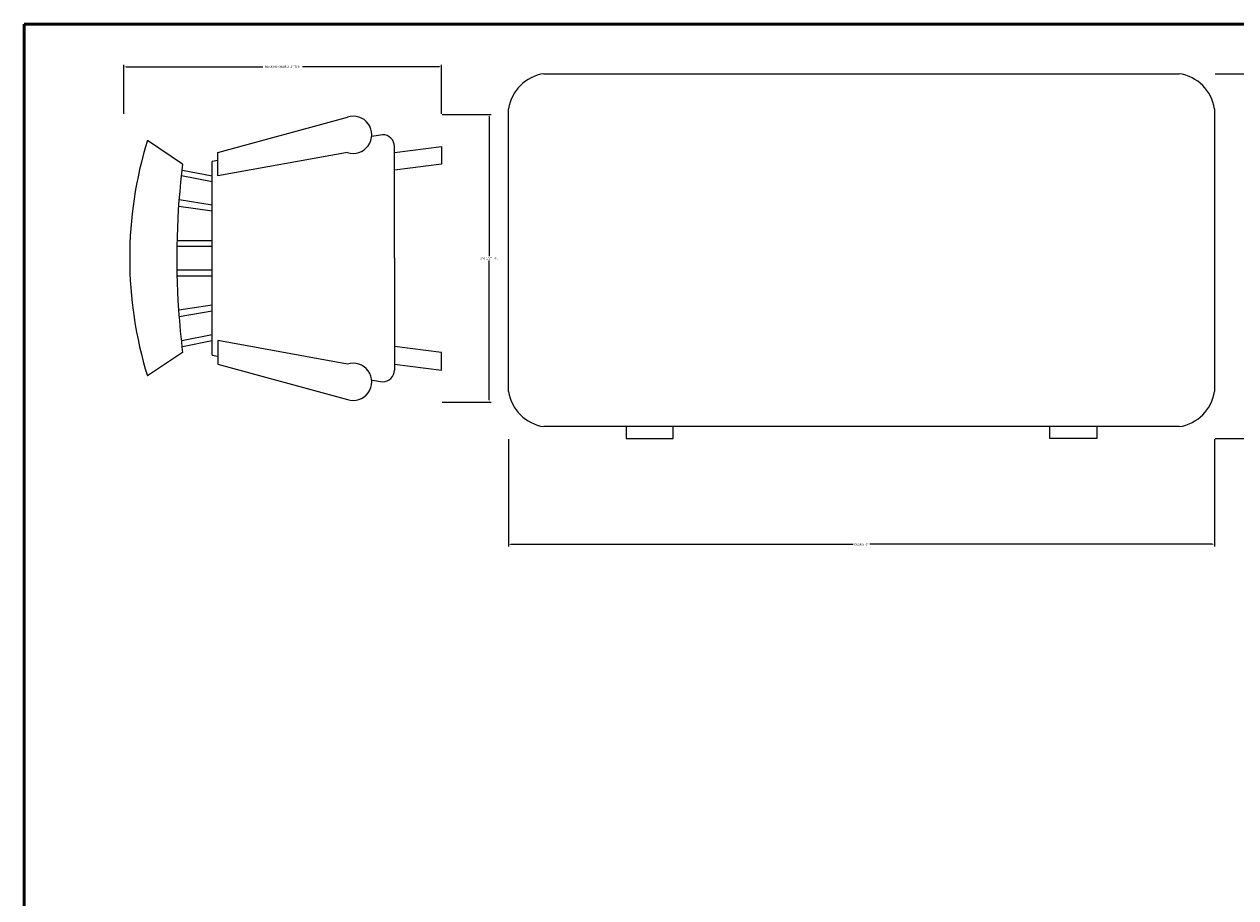
# Model space of a CAD drawing. Units: inches. Extents: x -105 to 1196, y -792 to 119.
# Tile 20 of 23: x 324 to 427, y -199 to -125. Entities that reach past the tile are written whole.
import ezdxf

# ---------------------------------------------------------------- set-up
doc = ezdxf.new("R2010")
doc.units = ezdxf.units.IN
doc.header["$MEASUREMENT"] = 0
for name, color, linetype, lineweight in [('A-ANNO-DIMS', 2, 'Continuous', 18), ('A-FURN', 8, 'Continuous', 18), ('A-WALL', 3, 'Continuous', 50)]:
    doc.layers.add(name, color=color, linetype=linetype, lineweight=lineweight)
doc.styles.get("Standard").update_dxf_attribs({"font": 'arial.ttf'})
doc.dimstyles.get("Standard").update_dxf_attribs({"dimtxt": 0.18, "dimasz": 0.18, "dimexe": 0.18, "dimexo": 0.0625, "dimgap": 0.09, "dimtad": 0, "dimtih": 1, "dimtoh": 1, "dimdec": 1, "dimzin": 0, "dimdsep": 46, "dimlunit": 4, "dimtxsty": 'Standard', "dimcen": 0.09, "dimadec": 0, "dimazin": 0, "dimtfac": 1, "dimtdec": 1, "dimtofl": 0, "dimtmove": 0, "dimatfit": 3, "dimfxl": 1, "dimtolj": 1, "dimtzin": 0, "dimarcsym": 0})

# ---------------------------------------------------------------- blocks, each defined once
blk = doc.blocks.new('Desk - 30 x 60 in.')
for p, q in [((-26.999995, 0), (26.999995, 0)), ((-29.999995, -27), (-29.999995, -3)), ((29.999995, -3), (29.999995, -27)), ((26.999995, -30), (-26.999995, -30)), ((-20.000005, -30), (-20.000005, -31)), ((-16.000005, -31), (-16.000005, -30)), ((15.999995, -31), (15.999995, -30)), ((19.999995, -30), (19.999995, -31)), ((-20.000005, -31), (-16.000005, -31)), ((19.999995, -31), (15.999995, -31))]:
    blk.add_line(p, q)
for centre, start, end in [((-26.499995, -3.5), 98.1301, 171.8699), ((26.499995, -3.5), 8.130102, 81.8699), ((-26.499995, -26.5), 188.1301, 261.8699), ((26.499995, -26.5), 278.1301, 351.8699)]:
    blk.add_arc(centre, 3.535534, start, end)
blk = doc.blocks.new('Chair - Rocking')
for p, q in [((-8, -4.5), (-10, -1.5)), ((8, -4.5), (10, -1.5)), ((-1.5, -4.05012), (-1.5, -7)), ((-1, -7), (-1, -4.05012)), ((1, -7), (1, -4.04655)), ((1.5, -4.05012), (1.5, -7)), ((-7.5, -4.5), (-7, -7)), ((-6.5, -7), (-7.02225, -4.43)), ((-4.5, -7), (-4.96674, -4.19951)), ((-4, -7), (-4.40532, -4.16272)), ((4, -7), (4.40187, -4.18694)), ((4.5, -7), (4.96761, -4.19437)), ((6.5, -7), (7, -4.4057)), ((7.5, -4.5), (7, -7)), ((-8.23428, -6.99939), (-8.3093, -7.47958)), ((-8.23041, -7), (8.23915, -7)), ((8.31071, -7.48854), (8.23449, -7.00073)), ((-9, -7.5), (-12, -18.49999)), ((-7, -7.5), (-9, -7.5)), ((-9, -18.49999), (-7, -7.5)), ((7, -7.5), (9, -7.5)), ((9, -18.49999), (7, -7.5)), ((9, -7.5), (12, -18.49999)), ((10.5, -21.49999), (10.3575, -20.58798)), ((-10.36644, -20.64523), (-10.5, -21.49999)), ((-9, -22.49999), (-9.5, -26.49999)), ((0, -22.49999), (-9.5, -22.49999)), ((-8, -26.49999), (-7.5, -22.49999)), ((0, -22.49999), (9.5, -22.49999)), ((8, -26.49999), (7.5, -22.49999)), ((9, -22.49999), (9.5, -26.49999)), ((-9.5, -26.49999), (-8, -26.49999)), ((9.5, -26.49999), (8, -26.49999))]:
    blk.add_line(p, q)
for centre, radius, start, end in [((0, -34.08333), 34.08333, 72.93847, 107.0615), ((0, -68.25004), 64.25, 82.84733, 93.92211), ((0, -68.25004), 64.25, 93.92211, 97.15267), ((-10.5, -18.99999), 1.58114, 161.5651, 18.43495), ((10.5, -18.99999), 1.58114, 161.5651, 18.43495), ((-9.5, -21.49999), 1, 180, 270), ((9.5, -21.49999), 1, 270, 0)]:
    blk.add_arc(centre, radius, start, end)
blk = doc.blocks.new('*D65')
at = {"layer": 'A-ANNO-DIMS', "color": 0, "lineweight": -2, "transparency": 16777216}
for p, q in [((332.21, -132.84), (332.21, -128.67)), ((359.21, -132.84), (359.21, -128.67)), ((332.39, -128.85), (344.03, -128.85)), ((359.03, -128.85), (347.4, -128.85))]:
    blk.add_line(p, q, dxfattribs=at)
at = {"layer": 'A-ANNO-DIMS', "color": 0, "transparency": 16777216}
for points in [[(332.39, -128.82), (332.39, -128.88), (332.21, -128.85)], [(359.03, -128.82), (359.03, -128.88), (359.21, -128.85)]]:
    blk.add_solid(points, dxfattribs=at)
at = {"layer": 'Defpoints', "color": 0, "transparency": 16777216}
for p in [(332.21, -128.85), (332.21, -132.9), (359.21, -132.9)]:
    blk.add_point(p, dxfattribs=at)
at = {"layer": 'A-ANNO-DIMS', "color": 0, "transparency": 16777216, "insert": (345.71, -128.85), "char_height": 0.18, "attachment_point": 5}
blk.add_mtext('\\A1;ROCKING CHAIR 2\'-3" TYP.', dxfattribs=at)
blk = doc.blocks.new('*D66')
at = {"layer": 'A-ANNO-DIMS', "color": 0, "lineweight": -2, "transparency": 16777216}
for p, q in [((359.28, -132.9), (363.44, -132.9)), ((363.26, -133.08), (363.26, -144.94)), ((363.26, -157.16), (363.26, -145.3)), ((359.28, -157.34), (363.44, -157.34))]:
    blk.add_line(p, q, dxfattribs=at)
at = {"layer": 'A-ANNO-DIMS', "color": 0, "transparency": 16777216}
for points in [[(363.23, -133.08), (363.29, -133.08), (363.26, -132.9)], [(363.23, -157.16), (363.29, -157.16), (363.26, -157.34)]]:
    blk.add_solid(points, dxfattribs=at)
at = {"layer": 'Defpoints', "color": 0, "transparency": 16777216}
for p in [(359.21, -132.9), (363.26, -132.9), (359.21, -157.34)]:
    blk.add_point(p, dxfattribs=at)
at = {"layer": 'A-ANNO-DIMS', "color": 0, "transparency": 16777216, "insert": (363.26, -145.12), "char_height": 0.18, "attachment_point": 5}
blk.add_mtext('\\A1;2\'-0 1/2" TYP.', dxfattribs=at)
blk = doc.blocks.new('*D73')
at = {"layer": 'A-ANNO-DIMS', "color": 0, "lineweight": -2, "transparency": 16777216}
for p, q in [((364.92, -160.49), (364.92, -169.61)), ((424.92, -160.49), (424.92, -169.61)), ((365.1, -169.43), (394.22, -169.43)), ((424.74, -169.43), (395.63, -169.43))]:
    blk.add_line(p, q, dxfattribs=at)
at = {"layer": 'A-ANNO-DIMS', "color": 0, "transparency": 16777216}
for points in [[(365.1, -169.4), (365.1, -169.46), (364.92, -169.43)], [(424.74, -169.4), (424.74, -169.46), (424.92, -169.43)]]:
    blk.add_solid(points, dxfattribs=at)
at = {"layer": 'Defpoints', "color": 0, "transparency": 16777216}
for p in [(364.92, -160.43), (424.92, -160.43), (424.92, -169.43)]:
    blk.add_point(p, dxfattribs=at)
at = {"layer": 'A-ANNO-DIMS', "color": 0, "transparency": 16777216, "insert": (394.92, -169.43), "char_height": 0.18, "attachment_point": 5}
blk.add_mtext('\\A1;DESK 5\'-0"', dxfattribs=at)
blk = doc.blocks.new('*D74')
at = {"layer": 'A-ANNO-DIMS', "color": 0, "lineweight": -2, "transparency": 16777216}
for p, q in [((424.99, -129.43), (434.1, -129.43)), ((433.92, -129.61), (433.92, -144.75)), ((433.92, -160.25), (433.92, -145.11)), ((424.99, -160.43), (434.1, -160.43))]:
    blk.add_line(p, q, dxfattribs=at)
at = {"layer": 'A-ANNO-DIMS', "color": 0, "transparency": 16777216}
for points in [[(433.89, -129.61), (433.95, -129.61), (433.92, -129.43)], [(433.89, -160.25), (433.95, -160.25), (433.92, -160.43)]]:
    blk.add_solid(points, dxfattribs=at)
at = {"layer": 'Defpoints', "color": 0, "transparency": 16777216}
for p in [(424.92, -129.43), (433.92, -129.43), (424.92, -160.43)]:
    blk.add_point(p, dxfattribs=at)
at = {"layer": 'A-ANNO-DIMS', "color": 0, "transparency": 16777216, "insert": (433.92, -144.93), "char_height": 0.18, "attachment_point": 5}
blk.add_mtext('\\A1;2\'-7"', dxfattribs=at)

msp = doc.modelspace()

# ---------------------------------------------------------------- linework, layer by layer
at = {"layer": 'A-WALL'}
for p, q in [((480.74, -125.23), (323.74, -125.23)), ((323.74, -125.23), (323.74, -228.23))]:
    msp.add_line(p, q, dxfattribs=at)

# ---------------------------------------------------------------- block references
at = {"layer": 'A-FURN'}
msp.add_blockref('Desk - 30 x 60 in.', (394.92, -129.43), dxfattribs=at)
at = {"layer": 'A-FURN', "rotation": 89.99999999999999}
msp.add_blockref('Chair - Rocking', (332.71, -145.12), dxfattribs=at)

# ---------------------------------------------------------------- dimensions: what is measured, and where the dimension line sits
at = {"layer": 'A-ANNO-DIMS'}
for base, p1, p2, angle, text, picture, middle in [((332.21, -128.85), (359.21, -132.9), (332.21, -132.9), 180, 'ROCKING CHAIR <> TYP.', '*D65', (345.71, -128.85)), ((363.26, -132.9), (359.21, -157.34), (359.21, -132.9), 90, '<> TYP.', '*D66', (363.26, -145.12))]:
    dim = msp.add_linear_dim(base=base, p1=p1, p2=p2, angle=angle, text=text, dimstyle='Standard', override={"dimdec": 1, "dimlfac": 1, "dimrnd": 0, "dimzin": 1, "dimdsep": 46, "dimlunit": 4, "dimfrac": 2}, dxfattribs=at)
    dim.commit()
    dim.dimension.update_dxf_attribs({"geometry": picture, "text_midpoint": middle})
dim = msp.add_linear_dim(base=(433.92, -129.43), p1=(424.92, -160.43), p2=(424.92, -129.43), angle=90, dimstyle='Standard', override={"dimdec": 1, "dimlfac": 1, "dimrnd": 0, "dimzin": 1, "dimdsep": 46, "dimlunit": 4, "dimfrac": 2}, dxfattribs=at)
dim.commit()
dim.dimension.update_dxf_attribs({"geometry": '*D74', "text_midpoint": (433.92, -144.93)})
dim = msp.add_linear_dim(base=(424.92, -169.43), p1=(364.92, -160.43), p2=(424.92, -160.43), text='DESK <>', dimstyle='Standard', override={"dimdec": 1, "dimlfac": 1, "dimrnd": 0, "dimzin": 1, "dimdsep": 46, "dimlunit": 4, "dimfrac": 2}, dxfattribs=at)
dim.commit()
dim.dimension.update_dxf_attribs({"geometry": '*D73', "text_midpoint": (394.92, -169.43)})

doc.saveas('drawing.dxf')
